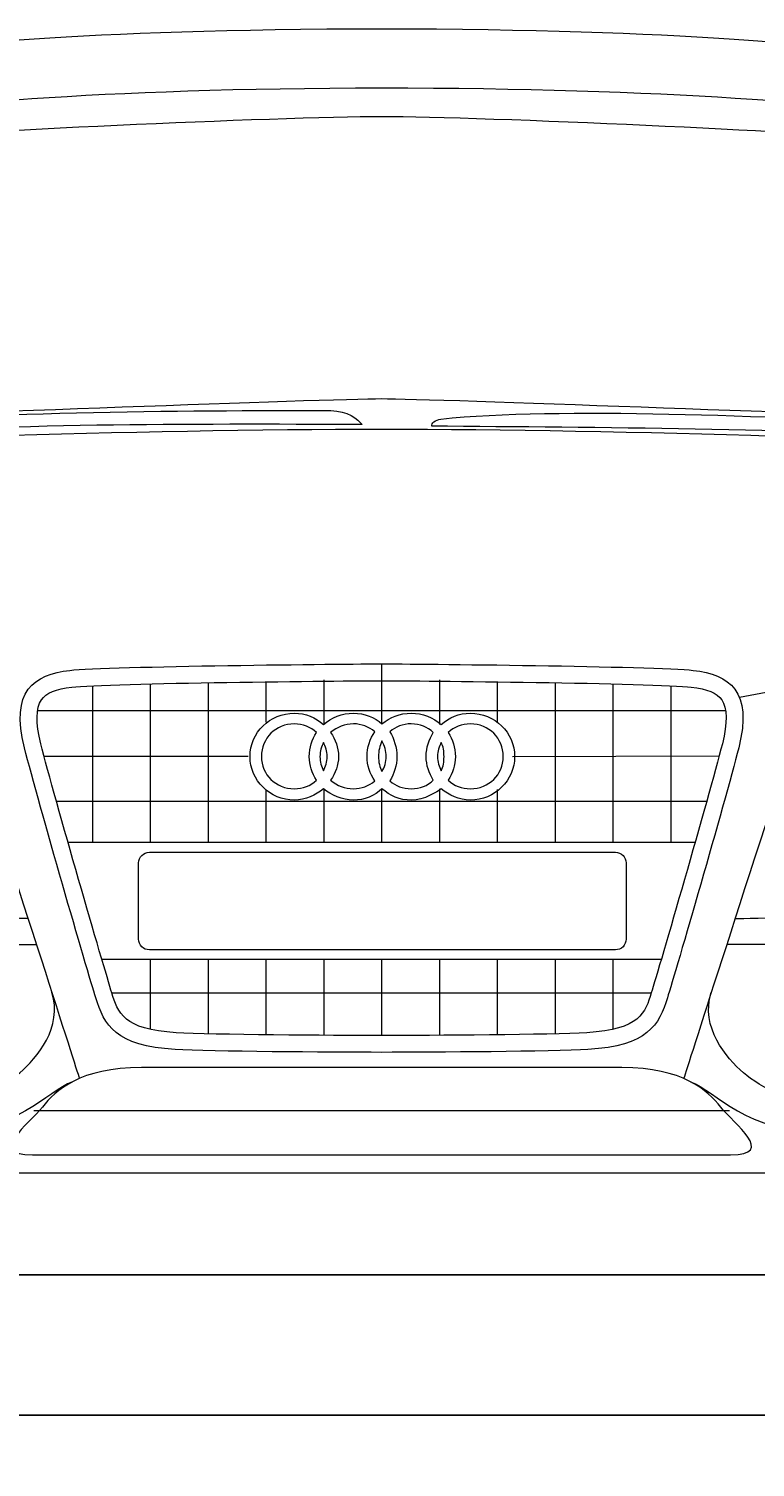
# Model space of a CAD drawing. Units: inches. Extents: x 1152 to 2588, y 1459 to 2618.
# Tile 10 of 17: x 1321 to 1352, y 2319 to 2381. Entities that reach past the tile are written whole.
import ezdxf

# ---------------------------------------------------------------- set-up
doc = ezdxf.new("R2010")
doc.units = ezdxf.units.IN
for name, color, linetype, lineweight in [('A-ANNO-DIMS', 2, 'Continuous', 18), ('A-ELEV', 7, 'Continuous', 25), ('AUDI', 7, 'Continuous', 13)]:
    doc.layers.add(name, color=color, linetype=linetype, lineweight=lineweight)
doc.styles.get("Standard").update_dxf_attribs({"font": 'arial.ttf'})
doc.dimstyles.get("Standard").update_dxf_attribs({"dimtxt": 0.18, "dimasz": 0.18, "dimexe": 0.18, "dimexo": 0.0625, "dimgap": 0.09, "dimtad": 0, "dimtih": 1, "dimtoh": 1, "dimdec": 4, "dimzin": 0, "dimdsep": 46, "dimtxsty": 'Standard', "dimcen": 0.09, "dimadec": 0, "dimazin": 0, "dimtfac": 1, "dimtdec": 4, "dimtofl": 0, "dimtmove": 0, "dimatfit": 3, "dimfxl": 1, "dimtolj": 1, "dimtzin": 0, "dimarcsym": 0})

# ---------------------------------------------------------------- blocks, each defined once
blk = doc.blocks.new('*D91')
at = {"layer": 'A-ANNO-DIMS', "color": 0, "lineweight": -2, "transparency": 16777216}
for p, q in [((1405.417, 2327.329), (1405.417, 2232.94)), ((1276.417, 2321.329), (1276.417, 2232.94)), ((1276.597, 2233.12), (1340.636, 2233.12)), ((1405.237, 2233.12), (1341.197, 2233.12))]:
    blk.add_line(p, q, dxfattribs=at)
at = {"layer": 'A-ANNO-DIMS', "color": 0, "transparency": 16777216}
for points in [[(1276.597, 2233.15), (1276.597, 2233.09), (1276.417, 2233.12)], [(1405.237, 2233.15), (1405.237, 2233.09), (1405.417, 2233.12)]]:
    blk.add_solid(points, dxfattribs=at)
at = {"layer": 'Defpoints', "color": 0, "transparency": 16777216}
for p in [(1405.417, 2327.391), (1276.417, 2321.391), (1405.417, 2233.12)]:
    blk.add_point(p, dxfattribs=at)
at = {"layer": 'A-ANNO-DIMS', "color": 0, "transparency": 16777216, "insert": (1340.917, 2233.12), "char_height": 0.18, "attachment_point": 5}
blk.add_mtext('\\A1;129', dxfattribs=at)

msp = doc.modelspace()

# ---------------------------------------------------------------- linework, layer by layer
at = {"layer": 'A-ELEV'}
for p, q in [((1736.4165, 2327.3911), (1285.4165, 2327.3911)), ((1736.4165, 2321.3911), (1276.4165, 2321.3911))]:
    msp.add_line(p, q, dxfattribs=at)
at = {"layer": 'AUDI'}
for points, knots in [([(1335.9514, 2380.6082), (1323.07, 2380.6082), (1316.2344, 2379.8209), (1314.9649, 2379.5565), (1314.9649, 2379.5565), (1313.6952, 2379.292), (1311.974, 2378.5979), (1310.5458, 2375.7943), (1310.5458, 2375.7943), (1309.1176, 2372.9909), (1306.1088, 2365.771), (1305.3217, 2364.6395), (1305.3217, 2364.6395), (1300.4024, 2362.1057), (1300.5918, 2357.8087), (1300.5428, 2357.4642), (1300.5428, 2357.4642), (1300.4936, 2357.1198), (1300.2995, 2356.5002), (1300.0824, 2356.2017), (1300.0824, 2356.2017), (1299.5785, 2355.5088), (1298.8858, 2353.5262), (1298.8858, 2352.3397), (1298.8858, 2352.3397), (1298.8858, 2347.9967), (1299.7554, 2343.0506), (1300.8566, 2337.73), (1300.8566, 2337.73), (1301.9224, 2332.5811), (1303.5104, 2331.7248), (1305.9177, 2331.7248), (1305.9177, 2331.7248), (1307.7191, 2331.725), (1335.9514, 2331.7248), (1335.9514, 2331.7248), (1335.9514, 2331.7248), (1335.9514, 2331.725), (1364.1837, 2331.7248), (1365.9852, 2331.7248), (1365.9852, 2331.7248), (1368.3925, 2331.725), (1369.9807, 2332.581), (1371.0466, 2337.73), (1371.0466, 2337.73), (1372.1483, 2343.0506), (1373.0181, 2347.9966), (1373.0181, 2352.3397), (1373.0181, 2352.3397), (1373.0181, 2353.5264), (1372.3251, 2355.5087), (1371.8212, 2356.2017), (1371.8212, 2356.2017), (1371.6039, 2356.5003), (1371.41, 2357.1198), (1371.3608, 2357.4642), (1371.3608, 2357.4642), (1371.3116, 2357.8087), (1371.501, 2362.1057), (1366.5811, 2364.6395), (1366.5811, 2364.6395), (1365.7941, 2365.7711), (1362.7853, 2372.9908), (1361.357, 2375.7943), (1361.357, 2375.7943), (1359.9288, 2378.5979), (1358.2076, 2379.292), (1356.9379, 2379.5565), (1356.9379, 2379.5565), (1355.6684, 2379.821), (1348.8329, 2380.608), (1335.9514, 2380.6082)], [0, 0, 0, 0, 0.0555556, 0.0555556, 0.0555556, 0.0555556, 0.1111111, 0.1111111, 0.1111111, 0.1111111, 0.1666667, 0.1666667, 0.1666667, 0.1666667, 0.2222222, 0.2222222, 0.2222222, 0.2222222, 0.2777778, 0.2777778, 0.2777778, 0.2777778, 0.3333333, 0.3333333, 0.3333333, 0.3333333, 0.3888889, 0.3888889, 0.3888889, 0.3888889, 0.4444444, 0.4444444, 0.4444444, 0.4444445, 0.5, 0.5, 0.5, 0.5, 0.5555556, 0.5555556, 0.5555556, 0.5555556, 0.6111111, 0.6111111, 0.6111111, 0.6111111, 0.6666667, 0.6666667, 0.6666667, 0.6666667, 0.7222222, 0.7222222, 0.7222222, 0.7222222, 0.7777778, 0.7777778, 0.7777778, 0.7777778, 0.8333333, 0.8333333, 0.8333333, 0.8333333, 0.8888889, 0.8888889, 0.8888889, 0.8888889, 0.9444444, 0.9444444, 0.9444444, 0.9444445, 1, 1, 1, 1]), ([(1335.9514, 2380.6082), (1323.07, 2380.6082), (1316.2344, 2379.8209), (1314.9649, 2379.5565), (1314.9649, 2379.5565), (1313.6952, 2379.292), (1311.974, 2378.5979), (1310.5458, 2375.7943), (1310.5458, 2375.7943), (1309.1176, 2372.9909), (1306.1088, 2365.771), (1305.3217, 2364.6395), (1305.3217, 2364.6395), (1300.4024, 2362.1057), (1300.5918, 2357.8087), (1300.5428, 2357.4642), (1300.5428, 2357.4642), (1300.4936, 2357.1198), (1300.2995, 2356.5002), (1300.0824, 2356.2017), (1300.0824, 2356.2017), (1299.5785, 2355.5088), (1298.8858, 2353.5262), (1298.8858, 2352.3397), (1298.8858, 2352.3397), (1298.8858, 2347.9967), (1299.7554, 2343.0506), (1300.8566, 2337.73), (1300.8566, 2337.73), (1301.9224, 2332.5811), (1303.5104, 2331.7248), (1305.9177, 2331.7248), (1305.9177, 2331.7248), (1307.7191, 2331.725), (1335.9514, 2331.7248), (1335.9514, 2331.7248), (1335.9514, 2331.7248), (1335.9514, 2331.7248), (1364.1837, 2331.7248), (1365.9852, 2331.7248), (1365.9852, 2331.7248), (1368.3925, 2331.725), (1369.9807, 2332.581), (1371.0466, 2337.73), (1371.0466, 2337.73), (1372.1483, 2343.0506), (1373.0181, 2347.9966), (1373.0181, 2352.3397), (1373.0181, 2352.3397), (1373.0181, 2353.5264), (1372.3251, 2355.5087), (1371.8212, 2356.2017), (1371.8212, 2356.2017), (1371.6039, 2356.5003), (1371.41, 2357.1198), (1371.3608, 2357.4642), (1371.3608, 2357.4642), (1371.3116, 2357.8087), (1371.501, 2362.1057), (1366.5811, 2364.6395), (1366.5811, 2364.6395), (1365.7941, 2365.7711), (1362.7853, 2372.9908), (1361.357, 2375.7943), (1361.357, 2375.7943), (1359.9288, 2378.5979), (1358.2076, 2379.292), (1356.9379, 2379.5565), (1356.9379, 2379.5565), (1355.6684, 2379.821), (1348.8329, 2380.608), (1335.9514, 2380.6082)], [0, 0, 0, 0, 0.0555556, 0.0555556, 0.0555556, 0.0555556, 0.1111111, 0.1111111, 0.1111111, 0.1111111, 0.1666667, 0.1666667, 0.1666667, 0.1666667, 0.2222222, 0.2222222, 0.2222222, 0.2222222, 0.2777778, 0.2777778, 0.2777778, 0.2777778, 0.3333333, 0.3333333, 0.3333333, 0.3333333, 0.3888889, 0.3888889, 0.3888889, 0.3888889, 0.4444444, 0.4444444, 0.4444444, 0.4444445, 0.5, 0.5, 0.5, 0.5, 0.5555556, 0.5555556, 0.5555556, 0.5555556, 0.6111111, 0.6111111, 0.6111111, 0.6111111, 0.6666667, 0.6666667, 0.6666667, 0.6666667, 0.7222222, 0.7222222, 0.7222222, 0.7222222, 0.7777778, 0.7777778, 0.7777778, 0.7777778, 0.8333333, 0.8333333, 0.8333333, 0.8333333, 0.8888889, 0.8888889, 0.8888889, 0.8888889, 0.9444444, 0.9444444, 0.9444444, 0.9444445, 1, 1, 1, 1]), ([(1335.9514, 2378.0831), (1323.862, 2378.0831), (1315.9013, 2377.3042), (1312.8453, 2376.7794), (1312.8453, 2376.7794), (1311.9763, 2375.2275), (1307.631, 2363.8673), (1307.5068, 2362.6256), (1307.5068, 2362.6256), (1310.8591, 2362.9982), (1325.7217, 2363.4947), (1335.9514, 2363.4947), (1335.9514, 2363.4947), (1346.1812, 2363.4947), (1361.0438, 2362.998), (1364.396, 2362.6256), (1364.396, 2362.6256), (1364.2719, 2363.8675), (1359.9266, 2375.2274), (1359.0575, 2376.7794), (1359.0575, 2376.7794), (1356.4376, 2377.3639), (1348.0408, 2378.0829), (1335.9514, 2378.0831)], [0, 0, 0, 0, 0.1666667, 0.1666667, 0.1666667, 0.1666667, 0.3333333, 0.3333333, 0.3333333, 0.3333333, 0.5, 0.5, 0.5, 0.5, 0.6666667, 0.6666667, 0.6666667, 0.6666667, 0.8333333, 0.8333333, 0.8333333, 0.8333333, 1, 1, 1, 1]), ([(1335.9514, 2376.8669), (1331.6617, 2376.8669), (1317.0146, 2376.1677), (1315.2481, 2375.9467), (1315.2481, 2375.9467), (1313.4816, 2375.7259), (1312.7088, 2374.9163), (1312.3775, 2373.8859), (1312.3775, 2373.8859), (1312.0463, 2372.8554), (1310.1695, 2368.1078), (1309.8383, 2367.0037), (1309.8383, 2367.0037), (1309.5071, 2365.8998), (1308.9561, 2363.9401), (1312.5985, 2364.0229), (1312.5985, 2364.0229), (1316.4298, 2364.1101), (1333.6902, 2364.7958), (1335.9514, 2364.7958), (1335.9514, 2364.7958), (1338.2126, 2364.7959), (1355.473, 2364.1101), (1359.3043, 2364.0229), (1359.3043, 2364.0229), (1362.9467, 2363.9401), (1362.3958, 2365.8997), (1362.0646, 2367.0037), (1362.0646, 2367.0037), (1361.7334, 2368.1079), (1359.8565, 2372.8554), (1359.5253, 2373.8859), (1359.5253, 2373.8859), (1359.1941, 2374.9164), (1358.4212, 2375.7259), (1356.6547, 2375.9467), (1356.6547, 2375.9467), (1354.8882, 2376.1677), (1340.2411, 2376.8668), (1335.9514, 2376.8669)], [0, 0, 0, 0, 0.1, 0.1, 0.1, 0.1, 0.2, 0.2, 0.2, 0.2, 0.3, 0.3, 0.3, 0.3, 0.4, 0.4, 0.4, 0.4, 0.5, 0.5, 0.5, 0.5, 0.6, 0.6, 0.6, 0.6, 0.7, 0.7, 0.7, 0.7, 0.8, 0.8, 0.8, 0.8, 0.9, 0.9, 0.9, 0.9, 1, 1, 1, 1]), ([(1333.7843, 2364.2972), (1327.6294, 2364.315), (1317.9085, 2364.2868), (1312.9628, 2363.5578), (1312.9628, 2363.5578), (1312.7186, 2363.5304), (1312.5333, 2363.3499), (1312.6234, 2363.227), (1312.6234, 2363.227), (1319.8823, 2363.7437), (1327.6218, 2363.7359), (1335.1175, 2363.7009), (1335.1175, 2363.7009), (1334.9378, 2363.9473), (1334.4852, 2364.288), (1333.7843, 2364.2972)], [0, 0, 0, 0, 0.25, 0.25, 0.25, 0.25, 0.5, 0.5, 0.5, 0.5, 0.75, 0.75, 0.75, 0.75, 1, 1, 1, 1]), ([(1333.7843, 2364.2972), (1327.6294, 2364.315), (1317.9085, 2364.2868), (1312.9628, 2363.5578), (1312.9628, 2363.5578), (1312.7186, 2363.5304), (1312.5333, 2363.3499), (1312.6234, 2363.227), (1312.6234, 2363.227), (1319.8823, 2363.7437), (1327.6218, 2363.7359), (1335.1175, 2363.7009), (1335.1175, 2363.7009), (1334.9378, 2363.9473), (1334.4852, 2364.288), (1333.7843, 2364.2972)], [0, 0, 0, 0, 0.25, 0.25, 0.25, 0.25, 0.5, 0.5, 0.5, 0.5, 0.75, 0.75, 0.75, 0.75, 1, 1, 1, 1]), ([(1333.7843, 2364.2972), (1327.6294, 2364.315), (1317.9085, 2364.2868), (1312.9628, 2363.5578), (1312.9628, 2363.5578), (1312.7186, 2363.5304), (1312.5333, 2363.3499), (1312.6234, 2363.227), (1312.6234, 2363.227), (1319.8823, 2363.7437), (1327.6218, 2363.7359), (1335.1175, 2363.7009), (1335.1175, 2363.7009), (1334.9378, 2363.9473), (1334.4852, 2364.288), (1333.7843, 2364.2972)], [0, 0, 0, 0, 0.25, 0.25, 0.25, 0.25, 0.5, 0.5, 0.5, 0.5, 0.75, 0.75, 0.75, 0.75, 1, 1, 1, 1]), ([(1360.6101, 2363.0565), (1360.4577, 2363.3307), (1359.6046, 2363.696), (1358.9039, 2363.7266), (1358.9039, 2363.7266), (1352.6576, 2364.0622), (1343.4864, 2364.4578), (1338.4895, 2363.9399), (1338.4895, 2363.9399), (1338.2456, 2363.9094), (1338.063, 2363.7572), (1338.0934, 2363.6353), (1338.0934, 2363.6353), (1345.3146, 2363.5742), (1353.4498, 2363.5438), (1360.4577, 2363.0868), (1360.4577, 2363.0868), (1360.5188, 2363.087), (1360.5491, 2363.0868), (1360.6101, 2363.0565)], [0, 0, 0, 0, 0.2, 0.2, 0.2, 0.2, 0.4, 0.4, 0.4, 0.4, 0.6, 0.6, 0.6, 0.6, 0.8, 0.8, 0.8, 0.8, 1, 1, 1, 1]), ([(1360.6101, 2363.0565), (1360.4577, 2363.3307), (1359.6046, 2363.696), (1358.9039, 2363.7266), (1358.9039, 2363.7266), (1352.6576, 2364.0622), (1343.4864, 2364.4578), (1338.4895, 2363.9399), (1338.4895, 2363.9399), (1338.2456, 2363.9094), (1338.063, 2363.7572), (1338.0934, 2363.6353), (1338.0934, 2363.6353), (1345.3146, 2363.5742), (1353.4498, 2363.5438), (1360.4577, 2363.0868), (1360.4577, 2363.0868), (1360.5188, 2363.087), (1360.5491, 2363.0868), (1360.6101, 2363.0565)], [0, 0, 0, 0, 0.2, 0.2, 0.2, 0.2, 0.4, 0.4, 0.4, 0.4, 0.6, 0.6, 0.6, 0.6, 0.8, 0.8, 0.8, 0.8, 1, 1, 1, 1]), ([(1360.6101, 2363.0565), (1360.4577, 2363.3307), (1359.6046, 2363.696), (1358.9039, 2363.7266), (1358.9039, 2363.7266), (1352.6576, 2364.0622), (1343.4864, 2364.4578), (1338.4895, 2363.9399), (1338.4895, 2363.9399), (1338.2456, 2363.9094), (1338.063, 2363.7572), (1338.0934, 2363.6353), (1338.0934, 2363.6353), (1345.3146, 2363.5742), (1353.4498, 2363.5438), (1360.4577, 2363.0868), (1360.4577, 2363.0868), (1360.5188, 2363.087), (1360.5491, 2363.0868), (1360.6101, 2363.0565)], [0, 0, 0, 0, 0.2, 0.2, 0.2, 0.2, 0.4, 0.4, 0.4, 0.4, 0.6, 0.6, 0.6, 0.6, 0.8, 0.8, 0.8, 0.8, 1, 1, 1, 1]), ([(1306.4516, 2362.6256), (1308.2711, 2362.0587), (1315.536, 2358.8847), (1318.1455, 2350.9148), (1318.1455, 2350.9148), (1320.7551, 2342.9449), (1323.0393, 2335.7729), (1323.0393, 2335.7729)], [0, 0, 0, 0, 0.5, 0.5, 0.5, 0.5, 1, 1, 1, 1]), ([(1365.4513, 2362.6256), (1363.6317, 2362.0587), (1356.3668, 2358.8847), (1353.7573, 2350.9148), (1353.7573, 2350.9148), (1351.1478, 2342.9449), (1348.8633, 2335.7722), (1348.8633, 2335.7722)], [0, 0, 0, 0, 0.5, 0.5, 0.5, 0.5, 1, 1, 1, 1]), ([(1335.9514, 2353.4829), (1334.637, 2353.4829), (1324.1786, 2353.3822), (1322.6342, 2353.2057), (1322.6342, 2353.2057), (1321.0898, 2353.0293), (1320.0748, 2352.3234), (1320.6926, 2349.8963), (1320.6926, 2349.8963), (1321.3105, 2347.4694), (1323.3842, 2340.3645), (1323.7374, 2339.2174), (1323.7374, 2339.2174), (1324.0905, 2338.0701), (1324.5802, 2337.1609), (1327.1353, 2337.0109), (1327.1353, 2337.0109), (1328.6449, 2336.9224), (1333.7102, 2336.8908), (1335.9514, 2336.8908), (1335.9514, 2336.8908), (1338.1926, 2336.8909), (1343.2579, 2336.9224), (1344.7675, 2337.0109), (1344.7675, 2337.0109), (1347.3226, 2337.1611), (1347.8123, 2338.0701), (1348.1655, 2339.2174), (1348.1655, 2339.2174), (1348.5186, 2340.3646), (1350.5923, 2347.4691), (1351.2102, 2349.8963), (1351.2102, 2349.8963), (1351.828, 2352.3236), (1350.813, 2353.0293), (1349.2687, 2353.2057), (1349.2687, 2353.2057), (1347.7244, 2353.3823), (1337.2658, 2353.4828), (1335.9514, 2353.4829)], [0, 0, 0, 0, 0.1, 0.1, 0.1, 0.1, 0.2, 0.2, 0.2, 0.2, 0.3, 0.3, 0.3, 0.3, 0.4, 0.4, 0.4, 0.4, 0.5, 0.5, 0.5, 0.5, 0.6, 0.6, 0.6, 0.6, 0.7, 0.7, 0.7, 0.7, 0.8, 0.8, 0.8, 0.8, 0.9, 0.9, 0.9, 0.9, 1, 1, 1, 1]), ([(1322.7158, 2352.4907), (1322.0412, 2352.4135), (1321.6165, 2352.2362), (1321.418, 2351.9481), (1321.418, 2351.9481), (1321.1766, 2351.5986), (1321.167, 2350.9503), (1321.3903, 2350.0738), (1321.3903, 2350.0738), (1321.9975, 2347.6879), (1324.079, 2340.5541), (1324.4252, 2339.4291), (1324.4252, 2339.4291), (1324.6841, 2338.5886), (1324.9073, 2337.8627), (1327.1774, 2337.7294), (1327.1774, 2337.7294), (1328.6915, 2337.6407), (1333.8368, 2337.6105), (1335.9514, 2337.6105), (1335.9514, 2337.6105), (1338.0661, 2337.6107), (1343.2115, 2337.6405), (1344.7254, 2337.7294), (1344.7254, 2337.7294), (1346.9953, 2337.8628), (1347.2189, 2338.5886), (1347.4776, 2339.4291), (1347.4776, 2339.4291), (1347.8239, 2340.5541), (1349.9053, 2347.6878), (1350.5125, 2350.0738), (1350.5125, 2350.0738), (1350.736, 2350.951), (1350.7262, 2351.5989), (1350.4848, 2351.9488), (1350.4848, 2351.9488), (1350.2862, 2352.2366), (1349.8617, 2352.4139), (1349.1873, 2352.4905), (1349.1873, 2352.4905), (1347.7054, 2352.6599), (1337.407, 2352.7631), (1335.9514, 2352.7631), (1335.9514, 2352.7631), (1334.496, 2352.7632), (1324.1974, 2352.6598), (1322.7158, 2352.4907)], [0, 0, 0, 0, 0.0833333, 0.0833333, 0.0833333, 0.0833333, 0.1666667, 0.1666667, 0.1666667, 0.1666667, 0.25, 0.25, 0.25, 0.25, 0.3333333, 0.3333333, 0.3333333, 0.3333333, 0.4166667, 0.4166667, 0.4166667, 0.4166667, 0.5, 0.5, 0.5, 0.5, 0.5833333, 0.5833333, 0.5833333, 0.5833333, 0.6666667, 0.6666667, 0.6666667, 0.6666667, 0.75, 0.75, 0.75, 0.75, 0.8333333, 0.8333333, 0.8333333, 0.8333333, 0.9166667, 0.9166667, 0.9166667, 0.9166667, 1, 1, 1, 1]), ([(1339.7466, 2351.3773), (1339.2592, 2351.3773), (1338.8327, 2351.1945), (1338.4975, 2350.8898), (1338.4975, 2350.8898), (1338.1625, 2351.1948), (1337.7053, 2351.3772), (1337.2177, 2351.3772), (1337.2177, 2351.3772), (1336.7303, 2351.3773), (1336.3037, 2351.1945), (1335.9686, 2350.9202), (1335.9686, 2350.9202), (1335.6642, 2351.1948), (1335.2067, 2351.3772), (1334.7498, 2351.3772), (1334.7498, 2351.3772), (1334.2622, 2351.3773), (1333.8051, 2351.1945), (1333.47, 2350.8898), (1333.47, 2350.8898), (1333.1348, 2351.1948), (1332.7084, 2351.3772), (1332.2209, 2351.3772), (1332.2209, 2351.3772), (1331.1848, 2351.3773), (1330.3316, 2350.5547), (1330.3316, 2349.5188), (1330.3316, 2349.5188), (1330.3316, 2348.5139), (1331.1848, 2347.6599), (1332.2209, 2347.6599), (1332.2209, 2347.6599), (1332.7084, 2347.6601), (1333.1348, 2347.8734), (1333.47, 2348.1476), (1333.47, 2348.1476), (1333.8051, 2347.8736), (1334.2622, 2347.6599), (1334.7498, 2347.6599), (1334.7498, 2347.6599), (1335.2067, 2347.6601), (1335.6642, 2347.843), (1335.9686, 2348.1476), (1335.9686, 2348.1476), (1336.3037, 2347.8431), (1336.7302, 2347.6599), (1337.2177, 2347.6599), (1337.2177, 2347.6599), (1337.7607, 2347.6601), (1338.3479, 2348.0252), (1338.4975, 2348.1476), (1338.4975, 2348.1476), (1338.8327, 2347.8736), (1339.2592, 2347.6599), (1339.7466, 2347.6599), (1339.7466, 2347.6599), (1340.7827, 2347.6601), (1341.6358, 2348.5137), (1341.6358, 2349.5188), (1341.6358, 2349.5188), (1341.6359, 2350.5547), (1340.7827, 2351.3772), (1339.7466, 2351.3773)], [0, 0, 0, 0, 0.0625, 0.0625, 0.0625, 0.0625, 0.125, 0.125, 0.125, 0.125, 0.1875, 0.1875, 0.1875, 0.1875, 0.25, 0.25, 0.25, 0.25, 0.3125, 0.3125, 0.3125, 0.3125, 0.375, 0.375, 0.375, 0.375, 0.4375, 0.4375, 0.4375, 0.4375, 0.5, 0.5, 0.5, 0.5, 0.5625, 0.5625, 0.5625, 0.5625, 0.625, 0.625, 0.625, 0.625, 0.6875, 0.6875, 0.6875, 0.6875, 0.75, 0.75, 0.75, 0.75, 0.8125, 0.8125, 0.8125, 0.8125, 0.875, 0.875, 0.875, 0.875, 0.9375, 0.9375, 0.9375, 0.9375, 1, 1, 1, 1]), ([(1339.7466, 2351.3773), (1339.2592, 2351.3773), (1338.8327, 2351.1945), (1338.4975, 2350.8898), (1338.4975, 2350.8898), (1338.1625, 2351.1948), (1337.7053, 2351.3772), (1337.2177, 2351.3772), (1337.2177, 2351.3772), (1336.7303, 2351.3773), (1336.3037, 2351.1945), (1335.9686, 2350.9202), (1335.9686, 2350.9202), (1335.6642, 2351.1948), (1335.2067, 2351.3772), (1334.7498, 2351.3772), (1334.7498, 2351.3772), (1334.2622, 2351.3773), (1333.8051, 2351.1945), (1333.47, 2350.8898), (1333.47, 2350.8898), (1333.1348, 2351.1948), (1332.7084, 2351.3772), (1332.2209, 2351.3772), (1332.2209, 2351.3772), (1331.1848, 2351.3773), (1330.3316, 2350.5547), (1330.3316, 2349.5188), (1330.3316, 2349.5188), (1330.3316, 2348.5139), (1331.1848, 2347.6599), (1332.2209, 2347.6599), (1332.2209, 2347.6599), (1332.7084, 2347.6601), (1333.1348, 2347.8734), (1333.47, 2348.1476), (1333.47, 2348.1476), (1333.8051, 2347.8736), (1334.2622, 2347.6599), (1334.7498, 2347.6599), (1334.7498, 2347.6599), (1335.2067, 2347.6601), (1335.6642, 2347.843), (1335.9686, 2348.1476), (1335.9686, 2348.1476), (1336.3037, 2347.8431), (1336.7302, 2347.6599), (1337.2177, 2347.6599), (1337.2177, 2347.6599), (1337.7607, 2347.6601), (1338.3479, 2348.0252), (1338.4975, 2348.1476), (1338.4975, 2348.1476), (1338.8327, 2347.8736), (1339.2592, 2347.6599), (1339.7466, 2347.6599), (1339.7466, 2347.6599), (1340.7827, 2347.6601), (1341.6358, 2348.5137), (1341.6358, 2349.5188), (1341.6358, 2349.5188), (1341.6358, 2350.5547), (1340.7827, 2351.3772), (1339.7466, 2351.3773)], [0, 0, 0, 0, 0.0625, 0.0625, 0.0625, 0.0625, 0.125, 0.125, 0.125, 0.125, 0.1875, 0.1875, 0.1875, 0.1875, 0.25, 0.25, 0.25, 0.25, 0.3125, 0.3125, 0.3125, 0.3125, 0.375, 0.375, 0.375, 0.375, 0.4375, 0.4375, 0.4375, 0.4375, 0.5, 0.5, 0.5, 0.5, 0.5625, 0.5625, 0.5625, 0.5625, 0.625, 0.625, 0.625, 0.625, 0.6875, 0.6875, 0.6875, 0.6875, 0.75, 0.75, 0.75, 0.75, 0.8125, 0.8125, 0.8125, 0.8125, 0.875, 0.875, 0.875, 0.875, 0.9375, 0.9375, 0.9375, 0.9375, 1, 1, 1, 1]), ([(1330.8193, 2349.5189), (1330.8193, 2350.3109), (1331.4287, 2350.9202), (1332.2209, 2350.9202), (1332.2209, 2350.9202), (1332.5864, 2350.9203), (1332.9215, 2350.7678), (1333.1654, 2350.5547), (1333.1654, 2350.5547), (1332.9826, 2350.25), (1332.8606, 2349.9147), (1332.8606, 2349.5188), (1332.8606, 2349.5188), (1332.8606, 2349.1531), (1332.9825, 2348.8179), (1333.1654, 2348.5137), (1333.1654, 2348.5137), (1332.9216, 2348.2697), (1332.5864, 2348.1476), (1332.2209, 2348.1476), (1332.2209, 2348.1476), (1331.4287, 2348.1476), (1330.8193, 2348.7569), (1330.8193, 2349.5189)], [0, 0, 0, 0, 0.1666667, 0.1666667, 0.1666667, 0.1666667, 0.3333333, 0.3333333, 0.3333333, 0.3333333, 0.5, 0.5, 0.5, 0.5, 0.6666667, 0.6666667, 0.6666667, 0.6666667, 0.8333333, 0.8333333, 0.8333333, 0.8333333, 1, 1, 1, 1]), ([(1333.7748, 2348.5139), (1333.9879, 2348.8179), (1334.1099, 2349.1531), (1334.1099, 2349.5188), (1334.1099, 2349.5188), (1334.1099, 2349.9148), (1333.9879, 2350.2498), (1333.7748, 2350.5547), (1333.7748, 2350.5547), (1334.0489, 2350.7679), (1334.384, 2350.9202), (1334.7498, 2350.9202), (1334.7498, 2350.9202), (1335.0851, 2350.9203), (1335.4201, 2350.7982), (1335.6642, 2350.585), (1335.6642, 2350.585), (1335.4506, 2350.2807), (1335.3286, 2349.9147), (1335.3286, 2349.5188), (1335.3286, 2349.5188), (1335.3286, 2349.1531), (1335.4506, 2348.7872), (1335.6642, 2348.4831), (1335.6642, 2348.4831), (1335.4202, 2348.2697), (1335.085, 2348.1476), (1334.7498, 2348.1476), (1334.7498, 2348.1476), (1334.384, 2348.1476), (1334.0489, 2348.2695), (1333.7748, 2348.5139)], [0, 0, 0, 0, 0.125, 0.125, 0.125, 0.125, 0.25, 0.25, 0.25, 0.25, 0.375, 0.375, 0.375, 0.375, 0.5, 0.5, 0.5, 0.5, 0.625, 0.625, 0.625, 0.625, 0.75, 0.75, 0.75, 0.75, 0.875, 0.875, 0.875, 0.875, 1, 1, 1, 1]), ([(1336.3037, 2348.4832), (1336.4867, 2348.7874), (1336.6083, 2349.1531), (1336.6083, 2349.5188), (1336.6083, 2349.5188), (1336.6083, 2349.9148), (1336.4865, 2350.2804), (1336.3037, 2350.585), (1336.3037, 2350.585), (1336.5474, 2350.7984), (1336.8522, 2350.9202), (1337.2177, 2350.9202), (1337.2177, 2350.9202), (1337.5834, 2350.9203), (1337.9186, 2350.7678), (1338.1623, 2350.5547), (1338.1623, 2350.5547), (1337.9795, 2350.25), (1337.8575, 2349.9147), (1337.8575, 2349.5188), (1337.8575, 2349.5188), (1337.8575, 2349.1531), (1337.9795, 2348.8179), (1338.1623, 2348.5137), (1338.1623, 2348.5137), (1337.9186, 2348.2697), (1337.5834, 2348.1476), (1337.2177, 2348.1476), (1337.2177, 2348.1476), (1336.8522, 2348.1476), (1336.5474, 2348.2695), (1336.3037, 2348.4832)], [0, 0, 0, 0, 0.125, 0.125, 0.125, 0.125, 0.25, 0.25, 0.25, 0.25, 0.375, 0.375, 0.375, 0.375, 0.5, 0.5, 0.5, 0.5, 0.625, 0.625, 0.625, 0.625, 0.75, 0.75, 0.75, 0.75, 0.875, 0.875, 0.875, 0.875, 1, 1, 1, 1]), ([(1339.7466, 2348.1476), (1339.3811, 2348.1476), (1339.0459, 2348.2695), (1338.8021, 2348.5137), (1338.8021, 2348.5137), (1338.985, 2348.8179), (1339.1069, 2349.1531), (1339.1069, 2349.5188), (1339.1069, 2349.5188), (1339.1069, 2349.9148), (1338.985, 2350.2498), (1338.8021, 2350.5547), (1338.8021, 2350.5547), (1339.0459, 2350.7679), (1339.3811, 2350.9202), (1339.7466, 2350.9202), (1339.7466, 2350.9202), (1340.5389, 2350.9203), (1341.1482, 2350.3108), (1341.1482, 2349.5188), (1341.1482, 2349.5188), (1341.1482, 2348.757), (1340.5388, 2348.1476), (1339.7466, 2348.1476)], [0, 0, 0, 0, 0.1666667, 0.1666667, 0.1666667, 0.1666667, 0.3333333, 0.3333333, 0.3333333, 0.3333333, 0.5, 0.5, 0.5, 0.5, 0.6666667, 0.6666667, 0.6666667, 0.6666667, 0.8333333, 0.8333333, 0.8333333, 0.8333333, 1, 1, 1, 1]), ([(1333.3176, 2349.5189), (1333.3176, 2349.7629), (1333.3787, 2349.9453), (1333.47, 2350.128), (1333.47, 2350.128), (1333.5615, 2349.9455), (1333.6224, 2349.7628), (1333.6224, 2349.5188), (1333.6224, 2349.5188), (1333.6224, 2349.3054), (1333.5615, 2349.0921), (1333.47, 2348.9092), (1333.47, 2348.9092), (1333.3787, 2349.0921), (1333.3176, 2349.3053), (1333.3176, 2349.5189)], [0, 0, 0, 0, 0.25, 0.25, 0.25, 0.25, 0.5, 0.5, 0.5, 0.5, 0.75, 0.75, 0.75, 0.75, 1, 1, 1, 1]), ([(1335.8163, 2349.5189), (1335.8163, 2349.7629), (1335.877, 2349.9756), (1335.9686, 2350.189), (1335.9686, 2350.189), (1336.0906, 2349.9757), (1336.1514, 2349.7628), (1336.1514, 2349.5188), (1336.1514, 2349.5188), (1336.1515, 2349.3054), (1336.0904, 2349.0617), (1335.9686, 2348.8789), (1335.9686, 2348.8789), (1335.877, 2349.0619), (1335.8162, 2349.3053), (1335.8163, 2349.5189)], [0, 0, 0, 0, 0.25, 0.25, 0.25, 0.25, 0.5, 0.5, 0.5, 0.5, 0.75, 0.75, 0.75, 0.75, 1, 1, 1, 1]), ([(1335.8163, 2349.5189), (1335.8163, 2349.7629), (1335.877, 2349.9756), (1335.9686, 2350.189), (1335.9686, 2350.189), (1336.0906, 2349.9757), (1336.1514, 2349.7628), (1336.1514, 2349.5188), (1336.1514, 2349.5188), (1336.1514, 2349.3054), (1336.0904, 2349.0617), (1335.9686, 2348.8789), (1335.9686, 2348.8789), (1335.877, 2349.0619), (1335.8163, 2349.3053), (1335.8163, 2349.5189)], [0, 0, 0, 0, 0.25, 0.25, 0.25, 0.25, 0.5, 0.5, 0.5, 0.5, 0.75, 0.75, 0.75, 0.75, 1, 1, 1, 1]), ([(1338.345, 2349.5189), (1338.345, 2349.7629), (1338.406, 2349.9453), (1338.4975, 2350.128), (1338.4975, 2350.128), (1338.5889, 2349.9455), (1338.6193, 2349.7628), (1338.6193, 2349.5188), (1338.6193, 2349.5188), (1338.6193, 2349.3054), (1338.5889, 2349.0921), (1338.4975, 2348.9092), (1338.4975, 2348.9092), (1338.406, 2349.0921), (1338.345, 2349.3053), (1338.345, 2349.5189)], [0, 0, 0, 0, 0.25, 0.25, 0.25, 0.25, 0.5, 0.5, 0.5, 0.5, 0.75, 0.75, 0.75, 0.75, 1, 1, 1, 1]), ([(1326.0318, 2345.4398), (1325.7777, 2345.4398), (1325.5709, 2345.233), (1325.5709, 2344.9788), (1325.5709, 2344.9788), (1325.5709, 2344.9788), (1325.5709, 2341.7278), (1325.5709, 2341.7278), (1325.5709, 2341.7278), (1325.5709, 2341.4739), (1325.7777, 2341.267), (1326.0318, 2341.267), (1326.0318, 2341.267), (1326.0318, 2341.267), (1345.9421, 2341.267), (1345.9421, 2341.267), (1345.9421, 2341.267), (1346.1962, 2341.267), (1346.4027, 2341.4738), (1346.4027, 2341.7277), (1346.4027, 2341.7277), (1346.4027, 2341.7277), (1346.4027, 2344.979), (1346.4027, 2344.979), (1346.4027, 2344.979), (1346.4027, 2345.2332), (1346.1962, 2345.4398), (1345.9421, 2345.4398), (1345.9421, 2345.4398), (1345.9421, 2345.4398), (1326.0318, 2345.4398), (1326.0318, 2345.4398)], [0, 0, 0, 0, 0.125, 0.125, 0.125, 0.125, 0.25, 0.25, 0.25, 0.25, 0.375, 0.375, 0.375, 0.375, 0.5, 0.5, 0.5, 0.5, 0.625, 0.625, 0.625, 0.625, 0.75, 0.75, 0.75, 0.75, 0.875, 0.875, 0.875, 0.875, 1, 1, 1, 1]), ([(1320.8458, 2342.6054), (1320.8458, 2342.6054), (1305.8379, 2342.8919), (1304.6212, 2342.8919), (1304.6212, 2342.8919), (1303.4046, 2342.8919), (1303.0872, 2341.1463), (1303.0872, 2340.2999), (1303.0872, 2340.2999), (1303.0872, 2339.4536), (1303.1401, 2338.2368), (1303.1401, 2337.4963), (1303.1401, 2337.4963), (1303.1401, 2336.7559), (1303.193, 2335.1159), (1305.8379, 2335.0101), (1305.8379, 2335.0101), (1308.4827, 2334.9044), (1315.1479, 2334.7456), (1316.7348, 2334.6927), (1316.7348, 2334.6927), (1318.3218, 2334.6399), (1319.75, 2335.3804), (1320.4906, 2336.0151), (1320.4906, 2336.0151), (1321.2312, 2336.6499), (1322.3377, 2337.9711), (1321.8613, 2339.452)], [0, 0, 0, 0, 0.1428571, 0.1428571, 0.1428571, 0.1428572, 0.2857143, 0.2857143, 0.2857143, 0.2857143, 0.4285714, 0.4285714, 0.4285714, 0.4285714, 0.5714286, 0.5714286, 0.5714286, 0.5714286, 0.7142857, 0.7142857, 0.7142857, 0.7142857, 0.8571429, 0.8571429, 0.8571429, 0.8571429, 1, 1, 1, 1]), ([(1351.057, 2342.6054), (1351.057, 2342.6054), (1366.0649, 2342.8919), (1367.2816, 2342.8919), (1367.2816, 2342.8919), (1368.4983, 2342.8919), (1368.8156, 2341.1463), (1368.8156, 2340.2999), (1368.8156, 2340.2999), (1368.8156, 2339.4536), (1368.7627, 2338.2368), (1368.7627, 2337.4963), (1368.7627, 2337.4963), (1368.7627, 2336.7559), (1368.7098, 2335.1159), (1366.0649, 2335.0101), (1366.0649, 2335.0101), (1363.4201, 2334.9044), (1356.7549, 2334.7456), (1355.168, 2334.6927), (1355.168, 2334.6927), (1353.5811, 2334.6399), (1352.1528, 2335.3804), (1351.4122, 2336.0151), (1351.4122, 2336.0151), (1350.6717, 2336.6499), (1349.5651, 2337.9711), (1350.0415, 2339.452)], [0, 0, 0, 0, 0.1428571, 0.1428571, 0.1428571, 0.1428572, 0.2857143, 0.2857143, 0.2857143, 0.2857143, 0.4285714, 0.4285714, 0.4285714, 0.4285714, 0.5714286, 0.5714286, 0.5714286, 0.5714286, 0.7142857, 0.7142857, 0.7142857, 0.7142857, 0.8571429, 0.8571429, 0.8571429, 0.8571429, 1, 1, 1, 1]), ([(1335.9514, 2332.5064), (1335.9514, 2332.5064), (1323.0118, 2332.5064), (1321.0371, 2332.5064), (1321.0371, 2332.5064), (1319.0624, 2332.5064), (1320.896, 2333.8463), (1321.4603, 2334.5515), (1321.4603, 2334.5515), (1322.0246, 2335.257), (1323.0693, 2336.2444), (1325.6922, 2336.2444), (1325.6922, 2336.2444), (1328.3149, 2336.2444), (1335.9514, 2336.2444), (1335.9514, 2336.2444), (1335.9514, 2336.2444), (1335.9514, 2336.2444), (1343.5879, 2336.2444), (1346.2106, 2336.2444), (1346.2106, 2336.2444), (1348.8335, 2336.2444), (1349.8782, 2335.2569), (1350.4425, 2334.5515), (1350.4425, 2334.5515), (1351.0069, 2333.8463), (1352.8404, 2332.5064), (1350.8657, 2332.5064), (1350.8657, 2332.5064), (1348.891, 2332.5064), (1335.9514, 2332.5064), (1335.9514, 2332.5064)], [0, 0, 0, 0, 0.125, 0.125, 0.125, 0.125, 0.25, 0.25, 0.25, 0.25, 0.375, 0.375, 0.375, 0.375, 0.5, 0.5, 0.5, 0.5, 0.625, 0.625, 0.625, 0.625, 0.75, 0.75, 0.75, 0.75, 0.875, 0.875, 0.875, 0.875, 1, 1, 1, 1]), ([(1322.7487, 2335.6318), (1321.6014, 2335.2217), (1320.4906, 2333.4761), (1316.8935, 2333.4232), (1316.8935, 2333.4232), (1313.2965, 2333.3703), (1302.7789, 2332.9116), (1302.7789, 2332.9116)], [0, 0, 0, 0, 0.5, 0.5, 0.5, 0.5, 1, 1, 1, 1]), ([(1349.1541, 2335.6318), (1350.3014, 2335.2217), (1351.4122, 2333.4761), (1355.0093, 2333.4232), (1355.0093, 2333.4232), (1358.6063, 2333.3703), (1369.1239, 2332.9116), (1369.1239, 2332.9116)], [0, 0, 0, 0, 0.5, 0.5, 0.5, 0.5, 1, 1, 1, 1]), ([(1321.0889, 2334.4107), (1321.0889, 2334.4107), (1335.9514, 2334.4107), (1335.9514, 2334.4107), (1335.9514, 2334.4107), (1335.9514, 2334.4107), (1350.8139, 2334.4107), (1350.8139, 2334.4107)], [0, 0, 0, 0, 0.5, 0.5, 0.5, 0.5, 1, 1, 1, 1])]:
    msp.add_open_spline(points, degree=3, knots=knots, dxfattribs=at)
for points in [[(1335.9514, 2353.4829), (1335.9514, 2353.4829), (1335.9514, 2350.9203), (1335.9514, 2350.9203)], [(1356.7845, 2353.0848), (1356.7845, 2353.0848), (1351.2418, 2352.0479), (1351.2418, 2352.0479)], [(1323.5959, 2352.5485), (1323.5959, 2352.5485), (1323.5959, 2345.8627), (1323.5959, 2345.8627)], [(1326.0669, 2352.6273), (1326.0669, 2352.6273), (1326.0669, 2345.8627), (1326.0669, 2345.8627)], [(1328.5382, 2352.6769), (1328.5382, 2352.6769), (1328.5382, 2345.8627), (1328.5382, 2345.8627)], [(1331.0092, 2352.7149), (1331.0092, 2352.7149), (1331.0092, 2350.9943), (1331.0092, 2350.9943)], [(1333.4803, 2352.7976), (1333.4803, 2352.7976), (1333.4803, 2350.8898), (1333.4803, 2350.8898)], [(1338.4225, 2352.7976), (1338.4225, 2352.7976), (1338.4225, 2350.8898), (1338.4225, 2350.8898)], [(1340.8936, 2352.7149), (1340.8936, 2352.7149), (1340.8936, 2350.9943), (1340.8936, 2350.9943)], [(1343.3648, 2352.6769), (1343.3648, 2352.6769), (1343.3648, 2345.8627), (1343.3648, 2345.8627)], [(1345.8359, 2352.6273), (1345.8359, 2352.6273), (1345.8359, 2345.8627), (1345.8359, 2345.8627)], [(1348.307, 2352.5485), (1348.307, 2352.5485), (1348.307, 2345.8627), (1348.307, 2345.8627)], [(1321.2536, 2351.484), (1321.2536, 2351.484), (1350.6639, 2351.484), (1350.6639, 2351.484)], [(1321.5306, 2349.5363), (1321.5306, 2349.5363), (1330.2478, 2349.5363), (1330.2478, 2349.5363)], [(1350.3723, 2349.5363), (1350.3723, 2349.5363), (1341.552, 2349.5189), (1341.552, 2349.5189)], [(1322.0546, 2347.6246), (1322.0546, 2347.6246), (1349.847, 2347.6246), (1349.847, 2347.6246)], [(1331.0092, 2348.1206), (1331.0092, 2348.1206), (1331.0092, 2345.8627), (1331.0092, 2345.8627)], [(1333.4803, 2348.1476), (1333.4803, 2348.1476), (1333.4803, 2345.8627), (1333.4803, 2345.8627)], [(1335.9514, 2348.1476), (1335.9514, 2348.1476), (1335.9514, 2345.8627), (1335.9514, 2345.8627)], [(1338.4225, 2348.1476), (1338.4225, 2348.1476), (1338.4225, 2345.8627), (1338.4225, 2345.8627)], [(1340.8936, 2348.1206), (1340.8936, 2348.1206), (1340.8936, 2345.8627), (1340.8936, 2345.8627)], [(1322.5522, 2345.8627), (1322.5522, 2345.8627), (1349.3792, 2345.8627), (1349.3792, 2345.8627)], [(1318.3844, 2341.4908), (1318.3844, 2341.4908), (1321.1857, 2341.4908), (1321.1857, 2341.4908)], [(1353.5184, 2341.4908), (1353.5184, 2341.4908), (1350.7172, 2341.4908), (1350.7172, 2341.4908)], [(1323.9959, 2340.8718), (1323.9959, 2340.8718), (1347.9074, 2340.8718), (1347.9074, 2340.8718)], [(1326.0669, 2340.8718), (1326.0669, 2340.8718), (1326.0669, 2337.883), (1326.0669, 2337.883)], [(1328.5382, 2340.8718), (1328.5382, 2340.8718), (1328.5382, 2337.6856), (1328.5382, 2337.6856)], [(1331.0092, 2340.8718), (1331.0092, 2340.8718), (1331.0092, 2337.6404), (1331.0092, 2337.6404)], [(1333.4803, 2340.8718), (1333.4803, 2340.8718), (1333.4803, 2337.6191), (1333.4803, 2337.6191)], [(1335.9514, 2340.8716), (1335.9514, 2340.8716), (1335.9514, 2337.6107), (1335.9514, 2337.6107)], [(1338.4225, 2340.8718), (1338.4225, 2340.8718), (1338.4225, 2337.6191), (1338.4225, 2337.6191)], [(1340.8936, 2340.8718), (1340.8936, 2340.8718), (1340.8936, 2337.6404), (1340.8936, 2337.6404)], [(1343.3648, 2340.8718), (1343.3648, 2340.8718), (1343.3648, 2337.6856), (1343.3648, 2337.6856)], [(1345.8359, 2340.8718), (1345.8359, 2340.8718), (1345.8359, 2337.883), (1345.8359, 2337.883)], [(1324.4253, 2339.4293), (1324.4253, 2339.4293), (1347.4776, 2339.4293), (1347.4776, 2339.4293)]]:
    msp.add_open_spline(points, degree=3, dxfattribs=at)

# ---------------------------------------------------------------- dimensions: what is measured, and where the dimension line sits
at = {"layer": 'A-ANNO-DIMS'}
dim = msp.add_linear_dim(base=(1405.4165, 2233.12), p1=(1276.4165, 2321.3911), p2=(1405.4165, 2327.3911), dimstyle='Standard', override={"dimdec": 0, "dimlfac": 1, "dimrnd": 0, "dimzin": 0, "dimdsep": 46, "dimlunit": 2}, dxfattribs=at)
dim.commit()
dim.dimension.update_dxf_attribs({"geometry": '*D91', "text_midpoint": (1340.9165, 2233.12)})

doc.saveas('drawing.dxf')
